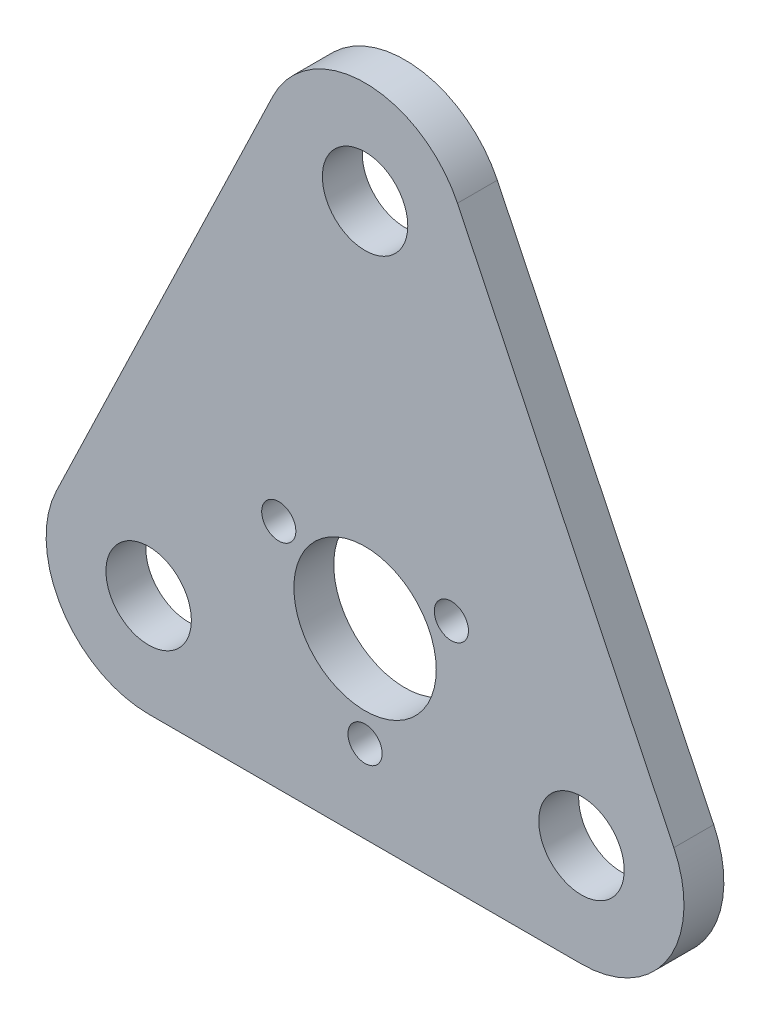
ISO-10303-21;
HEADER;
FILE_DESCRIPTION(('STEP AP214'),'2;1');
FILE_NAME('part.step','',(''),(''),'','','');
FILE_SCHEMA(('AUTOMOTIVE_DESIGN { 1 0 10303 214 1 1 1 1 }'));
ENDSEC;
DATA;
#1=APPLICATION_CONTEXT('core data for automotive mechanical design processes');
#2=APPLICATION_PROTOCOL_DEFINITION('international standard','automotive_design',2000,#1);
#3=PRODUCT_CONTEXT('',#1,'mechanical');
#4=PRODUCT('Part','Part','',(#3));
#5=PRODUCT_RELATED_PRODUCT_CATEGORY('part','',(#4));
#6=PRODUCT_DEFINITION_FORMATION('','',#4);
#7=PRODUCT_DEFINITION_CONTEXT('part definition',#1,'design');
#8=PRODUCT_DEFINITION('design','',#6,#7);
#9=PRODUCT_DEFINITION_SHAPE('','',#8);
#10=(LENGTH_UNIT() NAMED_UNIT(*) SI_UNIT(.MILLI.,.METRE.));
#11=(NAMED_UNIT(*) PLANE_ANGLE_UNIT() SI_UNIT($,.RADIAN.));
#12=(NAMED_UNIT(*) SI_UNIT($,.STERADIAN.) SOLID_ANGLE_UNIT());
#13=UNCERTAINTY_MEASURE_WITH_UNIT(LENGTH_MEASURE(1.E-05),#10,'distance_accuracy_value','');
#14=(GEOMETRIC_REPRESENTATION_CONTEXT(3) GLOBAL_UNCERTAINTY_ASSIGNED_CONTEXT((#13)) GLOBAL_UNIT_ASSIGNED_CONTEXT((#10,
#11,#12)) REPRESENTATION_CONTEXT('',''));
#15=CARTESIAN_POINT('',(0.,0.,0.));
#16=DIRECTION('',(0.,0.,1.));
#17=DIRECTION('',(1.,0.,0.));
#18=AXIS2_PLACEMENT_3D('',#15,#16,#17);
#19=CARTESIAN_POINT('',(-38.,-14.,7.));
#20=DIRECTION('',(0.,0.,1.));
#21=DIRECTION('',(1.,0.,0.));
#22=AXIS2_PLACEMENT_3D('',#19,#20,#21);
#23=PLANE('',#22);
#24=CARTESIAN_POINT('',(38.,-14.,7.));
#25=DIRECTION('',(0.,0.,1.));
#26=DIRECTION('',(-1.,0.,0.));
#27=AXIS2_PLACEMENT_3D('',#24,#25,#26);
#28=CIRCLE('',#27,7.50000000000001);
#29=CARTESIAN_POINT('',(30.5,-14.,7.));
#30=VERTEX_POINT('',#29);
#31=EDGE_CURVE('E212',#30,#30,#28,.T.);
#32=ORIENTED_EDGE('',*,*,#31,.F.);
#33=EDGE_LOOP('',(#32));
#34=FACE_BOUND('',#33,.T.);
#35=CARTESIAN_POINT('',(15.1554445662278,8.74999999999986,7.));
#36=DIRECTION('',(0.,0.,1.));
#37=DIRECTION('',(1.,0.,0.));
#38=AXIS2_PLACEMENT_3D('',#35,#36,#37);
#39=CIRCLE('',#38,3.);
#40=CARTESIAN_POINT('',(18.1554445662278,8.74999999999986,7.));
#41=VERTEX_POINT('',#40);
#42=EDGE_CURVE('E226',#41,#41,#39,.T.);
#43=ORIENTED_EDGE('',*,*,#42,.F.);
#44=EDGE_LOOP('',(#43));
#45=FACE_BOUND('',#44,.T.);
#46=CARTESIAN_POINT('',(0.,-17.5,7.));
#47=DIRECTION('',(0.,0.,1.));
#48=DIRECTION('',(1.,0.,0.));
#49=AXIS2_PLACEMENT_3D('',#46,#47,#48);
#50=CIRCLE('',#49,3.);
#51=CARTESIAN_POINT('',(3.,-17.5,7.));
#52=VERTEX_POINT('',#51);
#53=EDGE_CURVE('E236',#52,#52,#50,.T.);
#54=ORIENTED_EDGE('',*,*,#53,.F.);
#55=EDGE_LOOP('',(#54));
#56=FACE_BOUND('',#55,.T.);
#57=CARTESIAN_POINT('',(-38.,-14.,7.));
#58=DIRECTION('',(0.,0.,1.));
#59=DIRECTION('',(1.,0.,0.));
#60=AXIS2_PLACEMENT_3D('',#57,#58,#59);
#61=CIRCLE('',#60,18.);
#62=CARTESIAN_POINT('',(-54.2210013513531,-6.19749302086814,7.));
#63=VERTEX_POINT('',#62);
#64=CARTESIAN_POINT('',(-38.,-32.,7.));
#65=VERTEX_POINT('',#64);
#66=EDGE_CURVE('E143',#63,#65,#61,.T.);
#67=ORIENTED_EDGE('',*,*,#66,.T.);
#68=DIRECTION('',(1.,0.,0.));
#69=VECTOR('',#68,1.);
#70=CARTESIAN_POINT('',(-38.,-32.,7.));
#71=LINE('',#70,#69);
#72=CARTESIAN_POINT('',(38.,-32.,7.));
#73=VERTEX_POINT('',#72);
#74=EDGE_CURVE('E97',#65,#73,#71,.T.);
#75=ORIENTED_EDGE('',*,*,#74,.T.);
#76=CARTESIAN_POINT('',(38.,-14.,7.));
#77=DIRECTION('',(0.,0.,1.));
#78=DIRECTION('',(-1.,0.,0.));
#79=AXIS2_PLACEMENT_3D('',#76,#77,#78);
#80=CIRCLE('',#79,18.);
#81=CARTESIAN_POINT('',(54.2210013513531,-6.19749302086814,7.));
#82=VERTEX_POINT('',#81);
#83=EDGE_CURVE('E115',#73,#82,#80,.T.);
#84=ORIENTED_EDGE('',*,*,#83,.T.);
#85=DIRECTION('',(-0.43347260995177,0.901166741741838,0.));
#86=VECTOR('',#85,1.);
#87=CARTESIAN_POINT('',(54.2210013513531,-6.19749302086814,7.));
#88=LINE('',#87,#86);
#89=CARTESIAN_POINT('',(16.2210013513531,72.8025069791319,7.));
#90=VERTEX_POINT('',#89);
#91=EDGE_CURVE('E106',#82,#90,#88,.T.);
#92=ORIENTED_EDGE('',*,*,#91,.T.);
#93=CARTESIAN_POINT('',(0.,65.,7.));
#94=DIRECTION('',(0.,0.,1.));
#95=DIRECTION('',(1.,0.,0.));
#96=AXIS2_PLACEMENT_3D('',#93,#94,#95);
#97=CIRCLE('',#96,18.);
#98=CARTESIAN_POINT('',(-16.2210013513531,72.8025069791319,7.));
#99=VERTEX_POINT('',#98);
#100=EDGE_CURVE('E109',#90,#99,#97,.T.);
#101=ORIENTED_EDGE('',*,*,#100,.T.);
#102=DIRECTION('',(-0.43347260995177,-0.901166741741838,0.));
#103=VECTOR('',#102,1.);
#104=CARTESIAN_POINT('',(-54.2210013513531,-6.19749302086814,7.));
#105=LINE('',#104,#103);
#106=EDGE_CURVE('E65',#99,#63,#105,.T.);
#107=ORIENTED_EDGE('',*,*,#106,.T.);
#108=EDGE_LOOP('',(#67,#75,#84,#92,#101,#107));
#109=FACE_BOUND('',#108,.T.);
#110=CARTESIAN_POINT('',(0.,0.,7.));
#111=DIRECTION('',(0.,0.,1.));
#112=DIRECTION('',(1.,0.,0.));
#113=AXIS2_PLACEMENT_3D('',#110,#111,#112);
#114=CIRCLE('',#113,12.5);
#115=CARTESIAN_POINT('',(12.5,0.,7.));
#116=VERTEX_POINT('',#115);
#117=EDGE_CURVE('E133',#116,#116,#114,.T.);
#118=ORIENTED_EDGE('',*,*,#117,.F.);
#119=EDGE_LOOP('',(#118));
#120=FACE_BOUND('',#119,.T.);
#121=CARTESIAN_POINT('',(-15.1554445662276,8.75000000000007,7.));
#122=DIRECTION('',(0.,0.,1.));
#123=DIRECTION('',(1.,0.,0.));
#124=AXIS2_PLACEMENT_3D('',#121,#122,#123);
#125=CIRCLE('',#124,3.);
#126=CARTESIAN_POINT('',(-12.1554445662276,8.75000000000007,7.));
#127=VERTEX_POINT('',#126);
#128=EDGE_CURVE('E235',#127,#127,#125,.T.);
#129=ORIENTED_EDGE('',*,*,#128,.F.);
#130=EDGE_LOOP('',(#129));
#131=FACE_BOUND('',#130,.T.);
#132=CARTESIAN_POINT('',(-38.,-14.,7.));
#133=DIRECTION('',(0.,0.,1.));
#134=DIRECTION('',(1.,0.,0.));
#135=AXIS2_PLACEMENT_3D('',#132,#133,#134);
#136=CIRCLE('',#135,7.50000000000001);
#137=CARTESIAN_POINT('',(-30.5,-14.,7.));
#138=VERTEX_POINT('',#137);
#139=EDGE_CURVE('E219',#138,#138,#136,.T.);
#140=ORIENTED_EDGE('',*,*,#139,.F.);
#141=EDGE_LOOP('',(#140));
#142=FACE_BOUND('',#141,.T.);
#143=CARTESIAN_POINT('',(0.,65.,7.));
#144=DIRECTION('',(0.,0.,1.));
#145=DIRECTION('',(1.,0.,0.));
#146=AXIS2_PLACEMENT_3D('',#143,#144,#145);
#147=CIRCLE('',#146,7.50000000000001);
#148=CARTESIAN_POINT('',(7.50000000000001,65.,7.));
#149=VERTEX_POINT('',#148);
#150=EDGE_CURVE('E202',#149,#149,#147,.T.);
#151=ORIENTED_EDGE('',*,*,#150,.F.);
#152=EDGE_LOOP('',(#151));
#153=FACE_BOUND('',#152,.T.);
#154=ADVANCED_FACE('F44',(#34,#45,#56,#109,#120,#131,#142,#153),#23,.T.);
#155=CARTESIAN_POINT('',(-38.,-14.,0.));
#156=DIRECTION('',(0.,0.,1.));
#157=DIRECTION('',(1.,0.,0.));
#158=AXIS2_PLACEMENT_3D('',#155,#156,#157);
#159=PLANE('',#158);
#160=CARTESIAN_POINT('',(-38.,-14.,0.));
#161=DIRECTION('',(0.,0.,1.));
#162=DIRECTION('',(1.,0.,0.));
#163=AXIS2_PLACEMENT_3D('',#160,#161,#162);
#164=CIRCLE('',#163,18.);
#165=CARTESIAN_POINT('',(-54.2210013513531,-6.19749302086814,0.));
#166=VERTEX_POINT('',#165);
#167=CARTESIAN_POINT('',(-38.,-32.,0.));
#168=VERTEX_POINT('',#167);
#169=EDGE_CURVE('E128',#166,#168,#164,.T.);
#170=ORIENTED_EDGE('',*,*,#169,.F.);
#171=DIRECTION('',(-0.43347260995177,-0.901166741741838,0.));
#172=VECTOR('',#171,1.);
#173=CARTESIAN_POINT('',(-54.2210013513531,-6.19749302086814,0.));
#174=LINE('',#173,#172);
#175=CARTESIAN_POINT('',(-16.2210013513531,72.8025069791319,0.));
#176=VERTEX_POINT('',#175);
#177=EDGE_CURVE('E93',#176,#166,#174,.T.);
#178=ORIENTED_EDGE('',*,*,#177,.F.);
#179=CARTESIAN_POINT('',(0.,65.,0.));
#180=DIRECTION('',(0.,0.,1.));
#181=DIRECTION('',(1.,0.,0.));
#182=AXIS2_PLACEMENT_3D('',#179,#180,#181);
#183=CIRCLE('',#182,18.);
#184=CARTESIAN_POINT('',(16.2210013513531,72.8025069791319,0.));
#185=VERTEX_POINT('',#184);
#186=EDGE_CURVE('E84',#185,#176,#183,.T.);
#187=ORIENTED_EDGE('',*,*,#186,.F.);
#188=DIRECTION('',(-0.43347260995177,0.901166741741838,0.));
#189=VECTOR('',#188,1.);
#190=CARTESIAN_POINT('',(54.2210013513531,-6.19749302086814,0.));
#191=LINE('',#190,#189);
#192=CARTESIAN_POINT('',(54.2210013513531,-6.19749302086814,0.));
#193=VERTEX_POINT('',#192);
#194=EDGE_CURVE('E119',#193,#185,#191,.T.);
#195=ORIENTED_EDGE('',*,*,#194,.F.);
#196=CARTESIAN_POINT('',(38.,-14.,0.));
#197=DIRECTION('',(0.,0.,1.));
#198=DIRECTION('',(-1.,0.,0.));
#199=AXIS2_PLACEMENT_3D('',#196,#197,#198);
#200=CIRCLE('',#199,18.);
#201=CARTESIAN_POINT('',(38.,-32.,0.));
#202=VERTEX_POINT('',#201);
#203=EDGE_CURVE('E138',#202,#193,#200,.T.);
#204=ORIENTED_EDGE('',*,*,#203,.F.);
#205=DIRECTION('',(1.,0.,0.));
#206=VECTOR('',#205,1.);
#207=CARTESIAN_POINT('',(-38.,-32.,0.));
#208=LINE('',#207,#206);
#209=EDGE_CURVE('E132',#168,#202,#208,.T.);
#210=ORIENTED_EDGE('',*,*,#209,.F.);
#211=EDGE_LOOP('',(#170,#178,#187,#195,#204,#210));
#212=FACE_BOUND('',#211,.T.);
#213=CARTESIAN_POINT('',(0.,0.,0.));
#214=DIRECTION('',(0.,0.,1.));
#215=DIRECTION('',(1.,0.,0.));
#216=AXIS2_PLACEMENT_3D('',#213,#214,#215);
#217=CIRCLE('',#216,12.5);
#218=CARTESIAN_POINT('',(12.5,0.,0.));
#219=VERTEX_POINT('',#218);
#220=EDGE_CURVE('E241',#219,#219,#217,.T.);
#221=ORIENTED_EDGE('',*,*,#220,.T.);
#222=EDGE_LOOP('',(#221));
#223=FACE_BOUND('',#222,.T.);
#224=CARTESIAN_POINT('',(0.,-17.5,0.));
#225=DIRECTION('',(0.,0.,1.));
#226=DIRECTION('',(1.,0.,0.));
#227=AXIS2_PLACEMENT_3D('',#224,#225,#226);
#228=CIRCLE('',#227,3.);
#229=CARTESIAN_POINT('',(3.,-17.5,0.));
#230=VERTEX_POINT('',#229);
#231=EDGE_CURVE('E234',#230,#230,#228,.T.);
#232=ORIENTED_EDGE('',*,*,#231,.T.);
#233=EDGE_LOOP('',(#232));
#234=FACE_BOUND('',#233,.T.);
#235=CARTESIAN_POINT('',(-15.1554445662276,8.75000000000007,0.));
#236=DIRECTION('',(0.,0.,1.));
#237=DIRECTION('',(1.,0.,0.));
#238=AXIS2_PLACEMENT_3D('',#235,#236,#237);
#239=CIRCLE('',#238,3.);
#240=CARTESIAN_POINT('',(-12.1554445662276,8.75000000000007,0.));
#241=VERTEX_POINT('',#240);
#242=EDGE_CURVE('E228',#241,#241,#239,.T.);
#243=ORIENTED_EDGE('',*,*,#242,.T.);
#244=EDGE_LOOP('',(#243));
#245=FACE_BOUND('',#244,.T.);
#246=CARTESIAN_POINT('',(15.1554445662278,8.74999999999986,0.));
#247=DIRECTION('',(0.,0.,1.));
#248=DIRECTION('',(1.,0.,0.));
#249=AXIS2_PLACEMENT_3D('',#246,#247,#248);
#250=CIRCLE('',#249,3.);
#251=CARTESIAN_POINT('',(18.1554445662278,8.74999999999986,0.));
#252=VERTEX_POINT('',#251);
#253=EDGE_CURVE('E224',#252,#252,#250,.T.);
#254=ORIENTED_EDGE('',*,*,#253,.T.);
#255=EDGE_LOOP('',(#254));
#256=FACE_BOUND('',#255,.T.);
#257=CARTESIAN_POINT('',(-38.,-14.,0.));
#258=DIRECTION('',(0.,0.,1.));
#259=DIRECTION('',(1.,0.,0.));
#260=AXIS2_PLACEMENT_3D('',#257,#258,#259);
#261=CIRCLE('',#260,7.50000000000001);
#262=CARTESIAN_POINT('',(-30.5,-14.,0.));
#263=VERTEX_POINT('',#262);
#264=EDGE_CURVE('E220',#263,#263,#261,.T.);
#265=ORIENTED_EDGE('',*,*,#264,.T.);
#266=EDGE_LOOP('',(#265));
#267=FACE_BOUND('',#266,.T.);
#268=CARTESIAN_POINT('',(38.,-14.,0.));
#269=DIRECTION('',(0.,0.,1.));
#270=DIRECTION('',(-1.,0.,0.));
#271=AXIS2_PLACEMENT_3D('',#268,#269,#270);
#272=CIRCLE('',#271,7.50000000000001);
#273=CARTESIAN_POINT('',(30.5,-14.,0.));
#274=VERTEX_POINT('',#273);
#275=EDGE_CURVE('E211',#274,#274,#272,.T.);
#276=ORIENTED_EDGE('',*,*,#275,.T.);
#277=EDGE_LOOP('',(#276));
#278=FACE_BOUND('',#277,.T.);
#279=CARTESIAN_POINT('',(0.,65.,0.));
#280=DIRECTION('',(0.,0.,1.));
#281=DIRECTION('',(1.,0.,0.));
#282=AXIS2_PLACEMENT_3D('',#279,#280,#281);
#283=CIRCLE('',#282,7.50000000000001);
#284=CARTESIAN_POINT('',(7.50000000000001,65.,0.));
#285=VERTEX_POINT('',#284);
#286=EDGE_CURVE('E208',#285,#285,#283,.T.);
#287=ORIENTED_EDGE('',*,*,#286,.T.);
#288=EDGE_LOOP('',(#287));
#289=FACE_BOUND('',#288,.T.);
#290=ADVANCED_FACE('F147',(#212,#223,#234,#245,#256,#267,#278,#289),#159,.F.);
#291=CARTESIAN_POINT('',(-38.,-14.,7.));
#292=DIRECTION('',(0.,0.,-1.));
#293=DIRECTION('',(-1.,0.,0.));
#294=AXIS2_PLACEMENT_3D('',#291,#292,#293);
#295=CYLINDRICAL_SURFACE('',#294,18.);
#296=ORIENTED_EDGE('',*,*,#169,.T.);
#297=DIRECTION('',(0.,0.,-1.));
#298=VECTOR('',#297,1.);
#299=CARTESIAN_POINT('',(-38.,-32.,7.));
#300=LINE('',#299,#298);
#301=EDGE_CURVE('E11',#65,#168,#300,.T.);
#302=ORIENTED_EDGE('',*,*,#301,.F.);
#303=ORIENTED_EDGE('',*,*,#66,.F.);
#304=DIRECTION('',(0.,0.,-1.));
#305=VECTOR('',#304,1.);
#306=CARTESIAN_POINT('',(-54.2210013513531,-6.19749302086814,7.));
#307=LINE('',#306,#305);
#308=EDGE_CURVE('E127',#63,#166,#307,.T.);
#309=ORIENTED_EDGE('',*,*,#308,.T.);
#310=EDGE_LOOP('',(#296,#302,#303,#309));
#311=FACE_BOUND('',#310,.T.);
#312=ADVANCED_FACE('F50',(#311),#295,.T.);
#313=CARTESIAN_POINT('',(-38.,-32.,7.));
#314=DIRECTION('',(0.,1.,0.));
#315=DIRECTION('',(0.,0.,1.));
#316=AXIS2_PLACEMENT_3D('',#313,#314,#315);
#317=PLANE('',#316);
#318=ORIENTED_EDGE('',*,*,#209,.T.);
#319=DIRECTION('',(0.,0.,-1.));
#320=VECTOR('',#319,1.);
#321=CARTESIAN_POINT('',(38.,-32.,7.));
#322=LINE('',#321,#320);
#323=EDGE_CURVE('E53',#73,#202,#322,.T.);
#324=ORIENTED_EDGE('',*,*,#323,.F.);
#325=ORIENTED_EDGE('',*,*,#74,.F.);
#326=ORIENTED_EDGE('',*,*,#301,.T.);
#327=EDGE_LOOP('',(#318,#324,#325,#326));
#328=FACE_BOUND('',#327,.T.);
#329=ADVANCED_FACE('F386',(#328),#317,.F.);
#330=CARTESIAN_POINT('',(38.,-14.,7.));
#331=DIRECTION('',(0.,0.,-1.));
#332=DIRECTION('',(-1.,0.,0.));
#333=AXIS2_PLACEMENT_3D('',#330,#331,#332);
#334=CYLINDRICAL_SURFACE('',#333,18.);
#335=ORIENTED_EDGE('',*,*,#203,.T.);
#336=DIRECTION('',(0.,0.,-1.));
#337=VECTOR('',#336,1.);
#338=CARTESIAN_POINT('',(54.2210013513531,-6.19749302086814,7.));
#339=LINE('',#338,#337);
#340=EDGE_CURVE('E123',#82,#193,#339,.T.);
#341=ORIENTED_EDGE('',*,*,#340,.F.);
#342=ORIENTED_EDGE('',*,*,#83,.F.);
#343=ORIENTED_EDGE('',*,*,#323,.T.);
#344=EDGE_LOOP('',(#335,#341,#342,#343));
#345=FACE_BOUND('',#344,.T.);
#346=ADVANCED_FACE('F150',(#345),#334,.T.);
#347=CARTESIAN_POINT('',(54.2210013513531,-6.19749302086814,7.));
#348=DIRECTION('',(-0.901166741741838,-0.43347260995177,0.));
#349=DIRECTION('',(0.43347260995177,-0.901166741741838,0.));
#350=AXIS2_PLACEMENT_3D('',#347,#348,#349);
#351=PLANE('',#350);
#352=ORIENTED_EDGE('',*,*,#194,.T.);
#353=DIRECTION('',(0.,0.,-1.));
#354=VECTOR('',#353,1.);
#355=CARTESIAN_POINT('',(16.2210013513531,72.8025069791319,7.));
#356=LINE('',#355,#354);
#357=EDGE_CURVE('E120',#90,#185,#356,.T.);
#358=ORIENTED_EDGE('',*,*,#357,.F.);
#359=ORIENTED_EDGE('',*,*,#91,.F.);
#360=ORIENTED_EDGE('',*,*,#340,.T.);
#361=EDGE_LOOP('',(#352,#358,#359,#360));
#362=FACE_BOUND('',#361,.T.);
#363=ADVANCED_FACE('F117',(#362),#351,.F.);
#364=CARTESIAN_POINT('',(0.,65.,7.));
#365=DIRECTION('',(0.,0.,-1.));
#366=DIRECTION('',(-1.,0.,0.));
#367=AXIS2_PLACEMENT_3D('',#364,#365,#366);
#368=CYLINDRICAL_SURFACE('',#367,18.);
#369=ORIENTED_EDGE('',*,*,#186,.T.);
#370=DIRECTION('',(0.,0.,-1.));
#371=VECTOR('',#370,1.);
#372=CARTESIAN_POINT('',(-16.2210013513531,72.8025069791319,7.));
#373=LINE('',#372,#371);
#374=EDGE_CURVE('E125',#99,#176,#373,.T.);
#375=ORIENTED_EDGE('',*,*,#374,.F.);
#376=ORIENTED_EDGE('',*,*,#100,.F.);
#377=ORIENTED_EDGE('',*,*,#357,.T.);
#378=EDGE_LOOP('',(#369,#375,#376,#377));
#379=FACE_BOUND('',#378,.T.);
#380=ADVANCED_FACE('F122',(#379),#368,.T.);
#381=CARTESIAN_POINT('',(-54.2210013513531,-6.19749302086814,7.));
#382=DIRECTION('',(0.901166741741838,-0.43347260995177,0.));
#383=DIRECTION('',(0.43347260995177,0.901166741741838,0.));
#384=AXIS2_PLACEMENT_3D('',#381,#382,#383);
#385=PLANE('',#384);
#386=ORIENTED_EDGE('',*,*,#177,.T.);
#387=ORIENTED_EDGE('',*,*,#308,.F.);
#388=ORIENTED_EDGE('',*,*,#106,.F.);
#389=ORIENTED_EDGE('',*,*,#374,.T.);
#390=EDGE_LOOP('',(#386,#387,#388,#389));
#391=FACE_BOUND('',#390,.T.);
#392=ADVANCED_FACE('F154',(#391),#385,.F.);
#393=CARTESIAN_POINT('',(0.,0.,7.));
#394=DIRECTION('',(0.,0.,-1.));
#395=DIRECTION('',(-1.,0.,0.));
#396=AXIS2_PLACEMENT_3D('',#393,#394,#395);
#397=CYLINDRICAL_SURFACE('',#396,12.5);
#398=ORIENTED_EDGE('',*,*,#117,.T.);
#399=EDGE_LOOP('',(#398));
#400=FACE_BOUND('',#399,.T.);
#401=ORIENTED_EDGE('',*,*,#220,.F.);
#402=EDGE_LOOP('',(#401));
#403=FACE_BOUND('',#402,.T.);
#404=ADVANCED_FACE('F160',(#400,#403),#397,.F.);
#405=CARTESIAN_POINT('',(0.,-17.5,7.));
#406=DIRECTION('',(0.,0.,-1.));
#407=DIRECTION('',(-1.,0.,0.));
#408=AXIS2_PLACEMENT_3D('',#405,#406,#407);
#409=CYLINDRICAL_SURFACE('',#408,3.);
#410=ORIENTED_EDGE('',*,*,#53,.T.);
#411=EDGE_LOOP('',(#410));
#412=FACE_BOUND('',#411,.T.);
#413=ORIENTED_EDGE('',*,*,#231,.F.);
#414=EDGE_LOOP('',(#413));
#415=FACE_BOUND('',#414,.T.);
#416=ADVANCED_FACE('F163',(#412,#415),#409,.F.);
#417=CARTESIAN_POINT('',(-15.1554445662276,8.75000000000007,7.));
#418=DIRECTION('',(0.,0.,-1.));
#419=DIRECTION('',(-1.,0.,0.));
#420=AXIS2_PLACEMENT_3D('',#417,#418,#419);
#421=CYLINDRICAL_SURFACE('',#420,3.);
#422=ORIENTED_EDGE('',*,*,#128,.T.);
#423=EDGE_LOOP('',(#422));
#424=FACE_BOUND('',#423,.T.);
#425=ORIENTED_EDGE('',*,*,#242,.F.);
#426=EDGE_LOOP('',(#425));
#427=FACE_BOUND('',#426,.T.);
#428=ADVANCED_FACE('F179',(#424,#427),#421,.F.);
#429=CARTESIAN_POINT('',(15.1554445662278,8.74999999999986,7.));
#430=DIRECTION('',(0.,0.,-1.));
#431=DIRECTION('',(-1.,0.,0.));
#432=AXIS2_PLACEMENT_3D('',#429,#430,#431);
#433=CYLINDRICAL_SURFACE('',#432,3.);
#434=ORIENTED_EDGE('',*,*,#42,.T.);
#435=EDGE_LOOP('',(#434));
#436=FACE_BOUND('',#435,.T.);
#437=ORIENTED_EDGE('',*,*,#253,.F.);
#438=EDGE_LOOP('',(#437));
#439=FACE_BOUND('',#438,.T.);
#440=ADVANCED_FACE('F184',(#436,#439),#433,.F.);
#441=CARTESIAN_POINT('',(-38.,-14.,7.));
#442=DIRECTION('',(0.,0.,-1.));
#443=DIRECTION('',(-1.,0.,0.));
#444=AXIS2_PLACEMENT_3D('',#441,#442,#443);
#445=CYLINDRICAL_SURFACE('',#444,7.50000000000001);
#446=ORIENTED_EDGE('',*,*,#139,.T.);
#447=EDGE_LOOP('',(#446));
#448=FACE_BOUND('',#447,.T.);
#449=ORIENTED_EDGE('',*,*,#264,.F.);
#450=EDGE_LOOP('',(#449));
#451=FACE_BOUND('',#450,.T.);
#452=ADVANCED_FACE('F187',(#448,#451),#445,.F.);
#453=CARTESIAN_POINT('',(38.,-14.,7.));
#454=DIRECTION('',(0.,0.,-1.));
#455=DIRECTION('',(-1.,0.,0.));
#456=AXIS2_PLACEMENT_3D('',#453,#454,#455);
#457=CYLINDRICAL_SURFACE('',#456,7.50000000000001);
#458=ORIENTED_EDGE('',*,*,#31,.T.);
#459=EDGE_LOOP('',(#458));
#460=FACE_BOUND('',#459,.T.);
#461=ORIENTED_EDGE('',*,*,#275,.F.);
#462=EDGE_LOOP('',(#461));
#463=FACE_BOUND('',#462,.T.);
#464=ADVANCED_FACE('F195',(#460,#463),#457,.F.);
#465=CARTESIAN_POINT('',(0.,65.,7.));
#466=DIRECTION('',(0.,0.,-1.));
#467=DIRECTION('',(-1.,0.,0.));
#468=AXIS2_PLACEMENT_3D('',#465,#466,#467);
#469=CYLINDRICAL_SURFACE('',#468,7.50000000000001);
#470=ORIENTED_EDGE('',*,*,#150,.T.);
#471=EDGE_LOOP('',(#470));
#472=FACE_BOUND('',#471,.T.);
#473=ORIENTED_EDGE('',*,*,#286,.F.);
#474=EDGE_LOOP('',(#473));
#475=FACE_BOUND('',#474,.T.);
#476=ADVANCED_FACE('F198',(#472,#475),#469,.F.);
#477=CLOSED_SHELL('',(#154,#290,#312,#329,#346,#363,#380,#392,#404,#416,#428,#440,#452,#464,#476));
#478=MANIFOLD_SOLID_BREP('B2',#477);
#479=ADVANCED_BREP_SHAPE_REPRESENTATION('',(#18,#478),#14);
#480=SHAPE_DEFINITION_REPRESENTATION(#9,#479);
ENDSEC;
END-ISO-10303-21;
